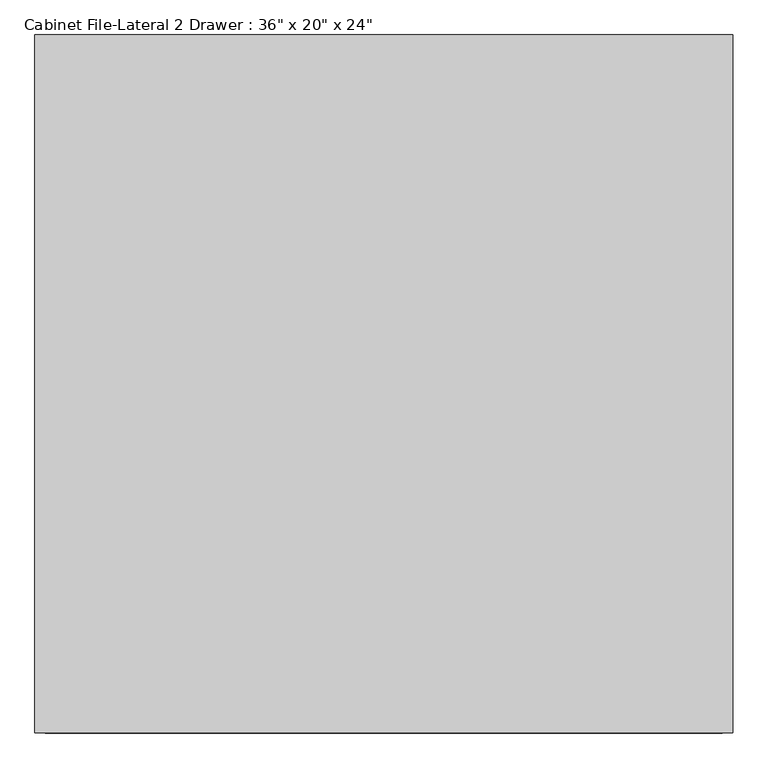
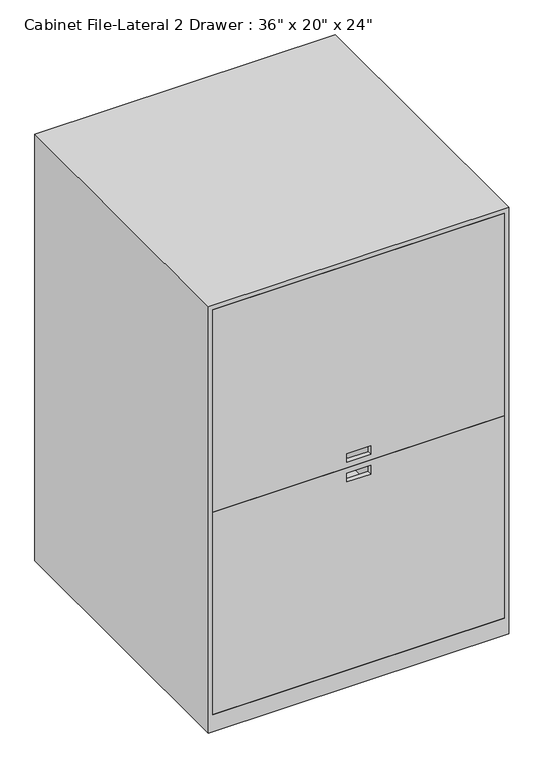
"""IFC4 building model written with IfcOpenShell, lengths in millimetres: furniture geometry."""

from ifc_helpers import new_model, si_unit, frame, origin, place, context, project, spatial, polyline, outline, extrude, faceted_brep, source, transform, mapped, element, save


def furniture_14b7b6c7(model_context):
    return source(origin(), model_context, "Body", "SolidModel", [
        faceted_brep([(454.9774861, -299.3183761, 1905.0), (-815.0225139, -299.3183761, 1905.0), (-815.0225139, -1569.3183761, 1905.0), (454.9774861, -1569.3183761, 1905.0), (454.9774861, -299.3183761, 0.0), (454.9774861, -1569.3183761, 0.0), (-815.0225139, -1569.3183761, 0.0), (-815.0225139, -299.3183761, 0.0), (435.9274861, -1569.3183761, 76.2), (-795.9725139, -1569.3183761, 76.2), (-795.9725139, -1569.3183761, 1885.95), (435.9274861, -1569.3183761, 1885.95), (-795.9725139, -318.3683761, 76.2), (435.9274861, -318.3683761, 76.2), (435.9274861, -318.3683761, 1885.95), (-795.9725139, -318.3683761, 1885.95)], [[[0, 1, 2, 3]], [[4, 5, 6, 7]], [[1, 0, 4, 7]], [[2, 1, 7, 6]], [[3, 2, 6, 5], [8, 9, 10, 11]], [[0, 3, 5, 4]], [[12, 13, 14, 15]], [[13, 12, 9, 8]], [[14, 13, 8, 11]], [[15, 14, 11, 10]], [[12, 15, 10, 9]]]),
        extrude(outline(polyline([(981.075, -795.9725139), (981.075, 435.9274861), (1885.95, 435.9274861), (1885.95, -795.9725139), (981.075, -795.9725139)]), holes=[polyline([(1044.575, -230.8225139), (1044.575, -129.2225139), (1006.475, -129.2225139), (1006.475, -230.8225139), (1044.575, -230.8225139)])]), frame((0.0, -1569.3183761, 0.0), z_axis=(0.0, 1.0, 0.0), x_axis=(0.0, 0.0, 1.0)), (0.0, 0.0, 1.0), 19.05),
        extrude(outline(polyline([(76.2, -795.9725139), (76.2, 435.9274861), (981.075, 435.9274861), (981.075, -795.9725139), (76.2, -795.9725139)]), holes=[polyline([(955.675, -230.8225139), (955.675, -129.2225139), (917.575, -129.2225139), (917.575, -230.8225139), (955.675, -230.8225139)])]), frame((0.0, -1569.3183761, 0.0), z_axis=(0.0, 1.0, 0.0), x_axis=(0.0, 0.0, 1.0)), (0.0, 0.0, 1.0), 19.05),
    ])


if __name__ == "__main__":
    model = new_model("IFC4")
    model_context = context("Model", 3, world=origin())
    ifc_project = project(units=[si_unit("LENGTHUNIT", "METRE", prefix="MILLI")], contexts=[model_context])
    site = spatial("IfcSite", under=ifc_project)
    building = spatial("IfcBuilding", under=site)
    placement = place(None, origin())
    furniture_shape = furniture_14b7b6c7(model_context)
    element("IfcFurniture", 1, ObjectType="Cabinet File-Lateral 2 Drawer : 36\" x 20\" x 24\"", at=placement, inside=building, context=model_context, shape_type="MappedRepresentation", body=[
        mapped(furniture_shape, transform((0.0, 0.0, 0.0), x_axis=(1.0, 0.0, 0.0), y_axis=(0.0, 1.0, 0.0), z_axis=(0.0, 0.0, 1.0))),
    ])
    save(model, "model.ifc")

# Revit data of these elements
# Type "Cabinet File-Lateral 2 Drawer : 36\" x 20\" x 24\""
#   Assembly Code = "E2020200"
#   Depth = 4' - 2"
#   Height = 6' - 3"
#   Width = 4' - 2"
#   Material = Metal - Steel
#   Default Elevation = 0
# Element 1 (IfcFurniture, "Cabinet File-Lateral 2 Drawer : 36\" x 20\" x 24\"")
#   Materials on its faces: "Metal - Steel"
# Materials
#   "Metal - Steel": colour RGB 210 210 210, transparency 0
